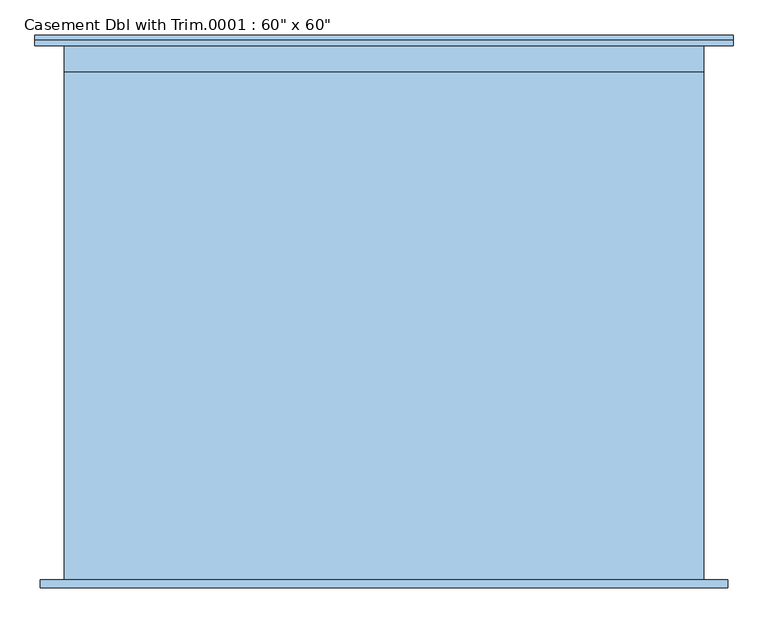
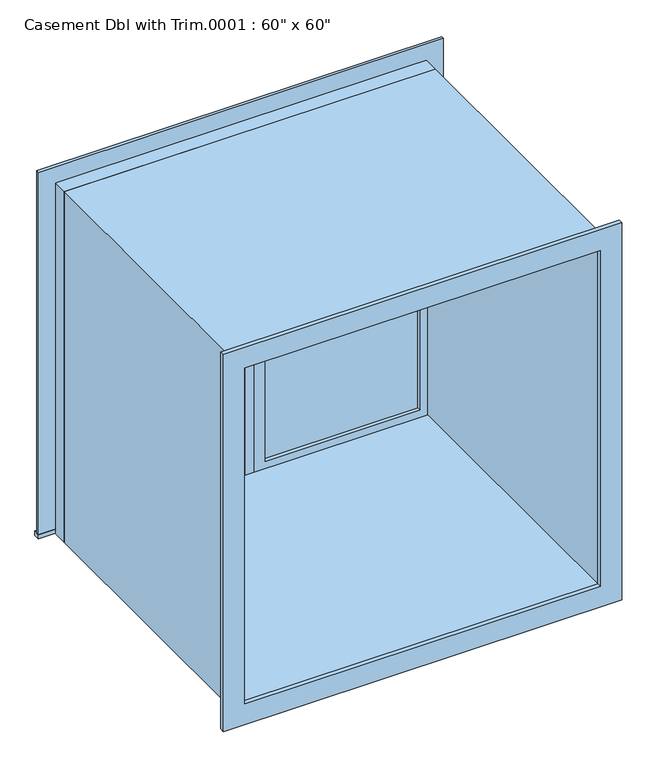
"""IFC4 building model written with IfcOpenShell, lengths in millimetres: window geometry."""

from ifc_helpers import new_model, si_unit, frame, origin, place, context, project, spatial, polyline, outline, extrude, source, transform, mapped, element, save


def window_0f4f1f5f(model_context):
    return source(origin(), model_context, "Body", "SweptSolid", [
        extrude(outline(polyline([(63.5, 621.1778585), (698.5, 621.1778585), (698.5, 608.4778585), (63.5, 608.4778585), (63.5, 621.1778585)])), frame((0.0, 0.0, 977.9), z_axis=(0.0, 0.0, 1.0), x_axis=(1.0, 0.0, 0.0)), (0.0, 0.0, 1.0), 1397.0),
        extrude(outline(polyline([(2419.35, 19.05), (933.45, 19.05), (933.45, 742.95), (2419.35, 742.95), (2419.35, 19.05)]), holes=[polyline([(2374.9, 63.5), (2374.9, 698.5), (977.9, 698.5), (977.9, 63.5), (2374.9, 63.5)])]), frame((0.0, 592.6028585, 0.0), z_axis=(0.0, 1.0, 0.0), x_axis=(0.0, 0.0, 1.0)), (0.0, 0.0, 1.0), 44.45),
        extrude(outline(polyline([(19.05, 592.6028585), (-19.05, 592.6028585), (-19.05, 656.1028585), (19.05, 656.1028585), (19.05, 592.6028585)])), frame((0.0, 0.0, 933.45), z_axis=(0.0, 0.0, 1.0), x_axis=(1.0, 0.0, 0.0)), (0.0, 0.0, 1.0), 1485.9),
        extrude(outline(polyline([(-831.85, 681.5028585), (831.85, 681.5028585), (831.85, 656.1028585), (-831.85, 656.1028585), (-831.85, 681.5028585)])), frame((0.0, 0.0, 914.4), z_axis=(0.0, 0.0, 1.0), x_axis=(1.0, 0.0, 0.0)), (0.0, 0.0, 1.0), 19.05),
        extrude(outline(polyline([(2419.35, -742.95), (2419.35, 742.95), (933.45, 742.95), (933.45, 831.85), (2508.25, 831.85), (2508.25, -831.85), (933.45, -831.85), (933.45, -742.95), (2419.35, -742.95)])), frame((0.0, 656.1028585, 0.0), z_axis=(0.0, 1.0, 0.0), x_axis=(0.0, 0.0, 1.0)), (0.0, 0.0, 1.0), 12.7),
        extrude(outline(polyline([(2495.55, 819.15), (2495.55, -819.15), (857.25, -819.15), (857.25, 819.15), (2495.55, 819.15)]), holes=[polyline([(2406.65, 730.25), (946.15, 730.25), (946.15, -730.25), (2406.65, -730.25), (2406.65, 730.25)])]), frame((0.0, -637.0528585, 0.0), z_axis=(0.0, 1.0, 0.0), x_axis=(0.0, 0.0, 1.0)), (0.0, 0.0, 1.0), 19.05),
        extrude(outline(polyline([(-63.5, 608.4778585), (-698.5, 608.4778585), (-698.5, 621.1778585), (-63.5, 621.1778585), (-63.5, 608.4778585)])), frame((0.0, 0.0, 977.9), z_axis=(0.0, 0.0, 1.0), x_axis=(1.0, 0.0, 0.0)), (0.0, 0.0, 1.0), 1397.0),
        extrude(outline(polyline([(2419.35, -742.95), (933.45, -742.95), (933.45, -19.05), (2419.35, -19.05), (2419.35, -742.95)]), holes=[polyline([(2374.9, -698.5), (2374.9, -63.5), (977.9, -63.5), (977.9, -698.5), (2374.9, -698.5)])]), frame((0.0, 592.6028585, 0.0), z_axis=(0.0, 1.0, 0.0), x_axis=(0.0, 0.0, 1.0)), (0.0, 0.0, 1.0), 44.45),
        extrude(outline(polyline([(2438.4, -762.0), (914.4, -762.0), (914.4, 762.0), (2438.4, 762.0), (2438.4, -762.0)]), holes=[polyline([(2406.65, -730.25), (2406.65, 730.25), (946.15, 730.25), (946.15, -730.25), (2406.65, -730.25)])]), frame((0.0, -618.0028585, 0.0), z_axis=(0.0, 1.0, 0.0), x_axis=(0.0, 0.0, 1.0)), (0.0, 0.0, 1.0), 1210.6057169),
        extrude(outline(polyline([(2438.4, 762.0), (2438.4, -762.0), (914.4, -762.0), (914.4, 762.0), (2438.4, 762.0)]), holes=[polyline([(2419.35, 742.95), (933.45, 742.95), (933.45, -742.95), (2419.35, -742.95), (2419.35, 742.95)])]), frame((0.0, 592.6028585, 0.0), z_axis=(0.0, 1.0, 0.0), x_axis=(0.0, 0.0, 1.0)), (0.0, 0.0, 1.0), 63.5),
    ])


if __name__ == "__main__":
    model = new_model("IFC4")
    model_context = context("Model", 3, world=origin())
    ifc_project = project(units=[si_unit("LENGTHUNIT", "METRE", prefix="MILLI")], contexts=[model_context])
    site = spatial("IfcSite", under=ifc_project)
    building = spatial("IfcBuilding", under=site)
    placement = place(None, origin())
    window_shape = window_0f4f1f5f(model_context)
    element("IfcWindow", 1, ObjectType="Casement Dbl with Trim.0001 : 60\" x 60\"", at=placement, inside=building, context=model_context, shape_type="MappedRepresentation", body=[
        mapped(window_shape, transform((0.0, 0.0, 0.0), x_axis=(1.0, 0.0, 0.0), y_axis=(0.0, 1.0, 0.0), z_axis=(0.0, 0.0, 1.0))),
    ])
    save(model, "model.ifc")

# Revit data of these elements
# Type "Casement Dbl with Trim.0001 : 60\" x 60\""
#   Type Mark = "10"
#   Construction Type Id = "GSP4R"
#   Assembly Code = "B2020100"
#   Analytic Construction = "1/8 in Pilkington single glazing"
#   Visual Light Transmittance = 0.9
#   Solar Heat Gain Coefficient = 0.78
#   Heat Transfer Coefficient (U) = 0.6496 BTU/(h·ft²·°F)
#   Height = 5' - 0"
#   Default Sill Height = 3' - 0"
#   Trim Projection - Ext. = 0' - 0 1/2"
#   Trim Projection - Int. = 0' - 0 3/4"
#   Trim Width - Exterior = 0' - 3 1/2"
#   Trim Width - Interior = 0' - 3 1/2"
#   Width = 5' - 0"
#   Window Inset = 0' - 0 3/4"
#   Define Thermal Properties by = 1
#   Glass Pane Material = Glass
#   Sash Material = Sash
#   Trim Exterior Material = Trim
#   Trim Interior Material = Trim
#   Wall Closure = (empty or 0)
# Element 1 (IfcWindow, "Casement Dbl with Trim.0001 : 60\" x 60\"")
#   Materials on its faces: "Sash", "Trim", "Glass"
# Materials
#   "Glass": class "Glass", colour RGB 0 128 192, transparency 0.75, Description = "Soda Lime Glass", Cost = 0
#   "Sash": class "Wood", colour RGB 224 178 126, transparency 0
#   "Trim": class "Wood", colour RGB 224 178 126, transparency 0
